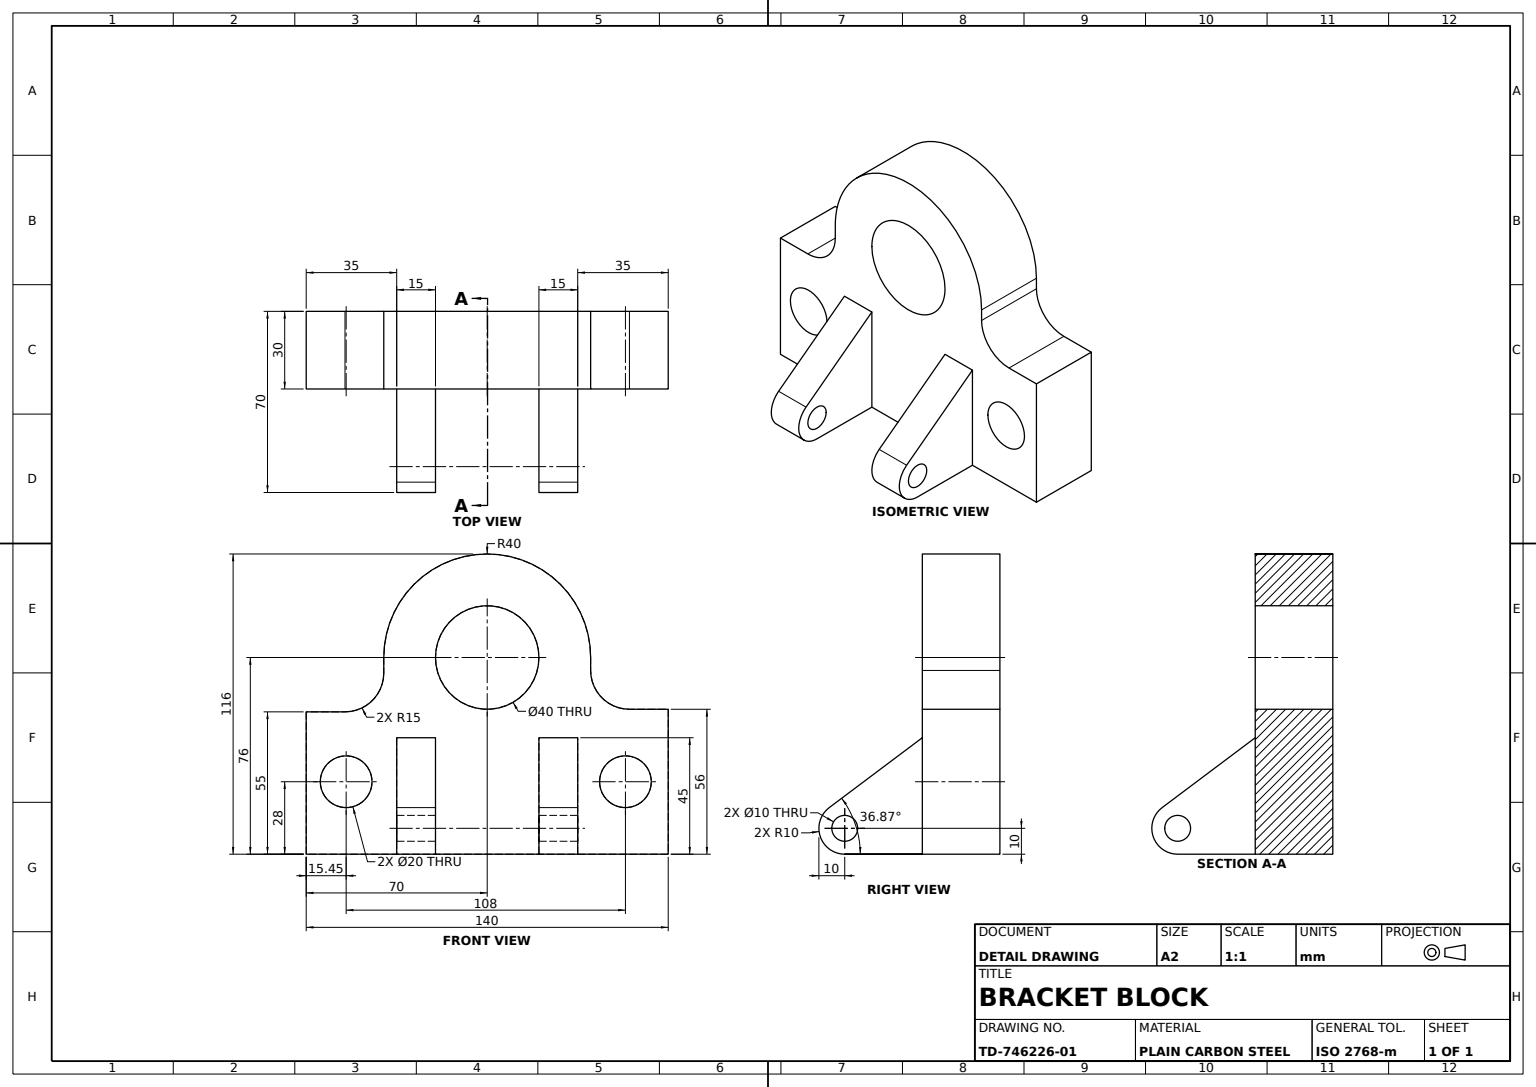
from build123d import *

# Parameters (mm, degrees)
BASE_PLATE_DEPTH         = 30
CENTER_BORE_PROFILE_R    = 20
CENTER_BORE_DEPTH        = 30
SIDE_HOLES_PROFILE_R     = 10
SIDE_HOLES_2X_28_DEPTH   = 30
LUG_1_DEPTH              = 50
LUG_1_TAPER_CUT_DEPTH    = 35
LUG_1_PIN_HOLE_PROFILE_R = 5
LUG_1_PIN_HOLE_DEPTH     = 15
LUG_START                = -50
LUG_2_DEPTH              = 50
LUG_START_2              = -35
LUG_2_TAPER_CUT_DEPTH    = 35
LUG_START_3              = -15
LUG_2_PIN_HOLE_PROFILE_R = 5
LUG_2_PIN_HOLE_DEPTH     = 15


with BuildPart() as part:
    # Base Plate Profile → Base Plate (new body)
    with BuildSketch(Plane.XY):
        with BuildLine():
            Line((0, 0), (140, 0))
            Line((140, 0), (140, 56))
            Line((140, 56), (125, 56))
            ThreePointArc((125, 56), (114.393398282, 60.393398282), (110, 71))
            Line((110, 71), (110, 76))
            ThreePointArc((110, 76), (70, 116), (30, 76))
            Line((30, 76), (30, 70))
            ThreePointArc((30, 70), (25.606601718, 59.393398282), (15, 55))
            Line((15, 55), (0, 55))
            Line((0, 55), (0, 0))
        make_face()
    extrude(amount=BASE_PLATE_DEPTH)

    # Center Bore Profile → Center Bore (cut)
    with BuildSketch(Plane.XY.offset(30)):
        with Locations((70, 76)):
            Circle(CENTER_BORE_PROFILE_R)
    extrude(amount=-CENTER_BORE_DEPTH, mode=Mode.SUBTRACT)

    # Side Holes Profile → Side Holes 2xØ28 (cut)
    with BuildSketch(Plane.XY.offset(30)):
        with Locations((15.451626978, 28)):
            Circle(SIDE_HOLES_PROFILE_R)
        with Locations((123.451626978, 28)):
            Circle(SIDE_HOLES_PROFILE_R)
    extrude(amount=-SIDE_HOLES_2X_28_DEPTH, mode=Mode.SUBTRACT)

    # Lug 1 Profile → Lug 1 (add)
    with BuildSketch(Plane.ZY):
        with BuildLine():
            Line((30, 0), (30, 45))
            Line((30, 45), (66, 18))
            ThreePointArc((66, 18), (69.486832981, 6.83772234), (60, 0))
            Line((60, 0), (30, 0))
        make_face()
    extrude(amount=-LUG_1_DEPTH)

    # Lug 1 Taper Profile → Lug 1 Taper Cut (cut)
    with BuildSketch(Plane.ZY):
        with BuildLine():
            Line((30, 45), (30, 0))
            Line((30, 0), (60, 0))
            ThreePointArc((60, 0), (69.486832981, 6.83772234), (66, 18))
            Line((66, 18), (30, 45))
        make_face()
    extrude(amount=-LUG_1_TAPER_CUT_DEPTH, mode=Mode.SUBTRACT)

    # Lug 1 Pin Hole Profile → Lug 1 Pin Hole (cut)
    with BuildSketch(Plane.ZY.offset(-35)):
        with Locations((60, 10)):
            Circle(LUG_1_PIN_HOLE_PROFILE_R)
    extrude(amount=-LUG_1_PIN_HOLE_DEPTH, mode=Mode.SUBTRACT)

    # Lug 2 Profile → Lug 2 (add)
    with BuildSketch(Plane(origin=(140, 0, 0), x_dir=(0, 0, -1), z_dir=(1, 0, 0)).offset(LUG_START)):
        with BuildLine():
            Line((-30, 0), (-30, 45))
            Line((-30, 45), (-66, 18))
            ThreePointArc((-66, 18), (-69.486832981, 6.83772234), (-60, 0))
            Line((-60, 0), (-30, 0))
        make_face()
    extrude(amount=LUG_2_DEPTH)

    # Lug 2 Taper Profile → Lug 2 Taper Cut (cut)
    with BuildSketch(Plane(origin=(140, 0, 0), x_dir=(0, 0, -1), z_dir=(1, 0, 0)).offset(LUG_START_2)):
        with BuildLine():
            Line((-30, 45), (-66, 18))
            ThreePointArc((-66, 18), (-69.486832981, 6.83772234), (-60, 0))
            Line((-60, 0), (-30, 0))
            Line((-30, 0), (-30, 45))
        make_face()
    extrude(amount=LUG_2_TAPER_CUT_DEPTH, mode=Mode.SUBTRACT)

    # Lug 2 Pin Hole Profile → Lug 2 Pin Hole (cut)
    with BuildSketch(Plane(origin=(105, 0, 0), x_dir=(0, 0, -1), z_dir=(1, 0, 0)).offset(LUG_START_3)):
        with Locations(Location((-60, 10, 0), (0, 0, 180))):
            Circle(LUG_2_PIN_HOLE_PROFILE_R)
    extrude(amount=LUG_2_PIN_HOLE_DEPTH, mode=Mode.SUBTRACT)


solid = part.part
